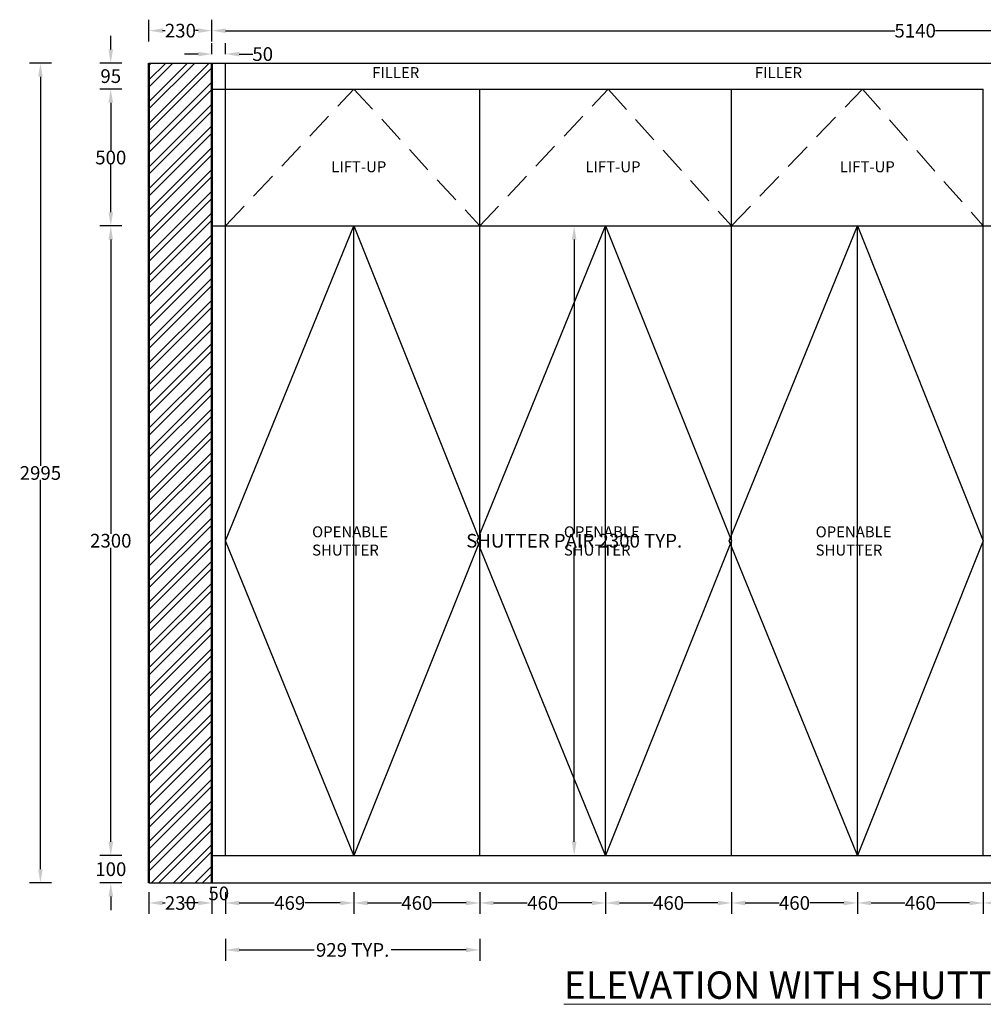
# Model space of a CAD drawing. Units: millimetres. Extents: x -472 to 16192, y -4730 to 4331.
# Tile 1 of 8: x -472 to 3049, y -4730 to -1132. Entities that reach past the tile are written whole.
import ezdxf

# ---------------------------------------------------------------- set-up
doc = ezdxf.new("R2010")
doc.units = ezdxf.units.MM
doc.header["$MEASUREMENT"] = 0
doc.linetypes.add('DASHED', pattern=[0.75, 0.5, -0.25])
for name, color, linetype, lineweight in [('A-ANNO-DIMS', 2, 'Continuous', 18), ('A-ANNO-TEXT', 6, 'Continuous', 18), ('A-ELEV', 7, 'Continuous', 25), ('A-ELEV-SWNG', 4, 'DASHED', 13), ('A-WALL', 7, 'Continuous', 50), ('A-WALL-PATT', 8, 'Continuous', 13)]:
    doc.layers.add(name, color=color, linetype=linetype, lineweight=lineweight)
doc.styles.get("Standard").update_dxf_attribs({"font": 'arial.ttf'})
doc.dimstyles.get("Standard").update_dxf_attribs({"dimtxt": 50, "dimasz": 50, "dimexe": 40, "dimexo": 40, "dimgap": 0.09, "dimtad": 0, "dimtih": 1, "dimtoh": 1, "dimdec": 0, "dimzin": 0, "dimdsep": 46, "dimtxsty": 'Standard', "dimcen": 0.09, "dimclrd": 1, "dimclre": 3, "dimclrt": 6, "dimadec": 0, "dimazin": 0, "dimtfac": 1, "dimtdec": 0, "dimtofl": 0, "dimtmove": 0, "dimatfit": 3, "dimfxl": 40, "dimfxlon": 1, "dimtolj": 1, "dimtzin": 0, "dimarcsym": 0})

# ---------------------------------------------------------------- blocks, each defined once
blk = doc.blocks.new('*D17')
at = {"layer": 'A-ANNO-DIMS', "color": 0, "lineweight": -2, "transparency": 16777216}
for p, q in [((230, -1212.4), (230, -1132.4)), ((5370, -1212.4), (5370, -1132.4)), ((280, -1172.4), (2725.3, -1172.4)), ((5320, -1172.4), (2874.7, -1172.4))]:
    blk.add_line(p, q, dxfattribs=at)
at = {"layer": 'A-ANNO-DIMS', "color": 0, "transparency": 16777216}
for points in [[(280, -1164.1), (280, -1180.8), (230, -1172.4)], [(5320, -1164.1), (5320, -1180.8), (5370, -1172.4)]]:
    blk.add_solid(points, dxfattribs=at)
at = {"layer": 'Defpoints', "color": 0, "transparency": 16777216}
for p in [(5370, -1172.4), (230, -1290.9), (5370, -1290.9)]:
    blk.add_point(p, dxfattribs=at)
at = {"layer": 'A-ANNO-DIMS', "color": 0, "transparency": 16777216, "insert": (2800, -1172.4), "char_height": 50, "attachment_point": 5}
blk.add_mtext('\\A1;5140', dxfattribs=at)
blk = doc.blocks.new('*D19')
at = {"layer": 'A-ANNO-DIMS', "color": 0, "lineweight": -2, "transparency": 16777216}
for p, q in [((230, -1257.8), (230, -1217.8)), ((280, -1257.8), (280, -1217.8)), ((180, -1257.8), (130, -1257.8)), ((330, -1257.8), (380, -1257.8))]:
    blk.add_line(p, q, dxfattribs=at)
at = {"layer": 'A-ANNO-DIMS', "color": 0, "transparency": 16777216}
for points in [[(180, -1249.5), (180, -1266.2), (230, -1257.8)], [(330, -1249.5), (330, -1266.2), (280, -1257.8)]]:
    blk.add_solid(points, dxfattribs=at)
at = {"layer": 'Defpoints', "color": 0, "transparency": 16777216}
for p in [(280, -1257.8), (230, -1290.9), (280, -1290.9)]:
    blk.add_point(p, dxfattribs=at)
at = {"layer": 'A-ANNO-DIMS', "color": 0, "transparency": 16777216, "insert": (415.8, -1257.8), "char_height": 50, "attachment_point": 5}
blk.add_mtext('\\A1;50', dxfattribs=at)
blk = doc.blocks.new('*D20')
at = {"layer": 'A-ANNO-DIMS', "color": 0, "lineweight": -2, "transparency": 16777216}
for p, q in [((0, -1212.3), (0, -1132.3)), ((230, -1212.3), (230, -1132.3)), ((50, -1172.3), (59.3, -1172.3)), ((180, -1172.3), (170.7, -1172.3))]:
    blk.add_line(p, q, dxfattribs=at)
at = {"layer": 'A-ANNO-DIMS', "color": 0, "transparency": 16777216}
for points in [[(50, -1163.9), (50, -1180.6), (0, -1172.3)], [(180, -1163.9), (180, -1180.6), (230, -1172.3)]]:
    blk.add_solid(points, dxfattribs=at)
at = {"layer": 'Defpoints', "color": 0, "transparency": 16777216}
for p in [(230, -1172.3), (0, -1290.9), (230, -1290.9)]:
    blk.add_point(p, dxfattribs=at)
at = {"layer": 'A-ANNO-DIMS', "color": 0, "transparency": 16777216, "insert": (115, -1172.3), "char_height": 50, "attachment_point": 5}
blk.add_mtext('\\A1;230', dxfattribs=at)
blk = doc.blocks.new('*D21')
at = {"layer": 'A-ANNO-DIMS', "color": 0, "lineweight": -2, "transparency": 16777216}
for p, q in [((-356.5, -1290.9), (-436.5, -1290.9)), ((-396.5, -1340.9), (-396.5, -2762.8)), ((-396.5, -4235.9), (-396.5, -2814)), ((-356.5, -4285.9), (-436.5, -4285.9))]:
    blk.add_line(p, q, dxfattribs=at)
at = {"layer": 'A-ANNO-DIMS', "color": 0, "transparency": 16777216}
for points in [[(-404.8, -1340.9), (-388.1, -1340.9), (-396.5, -1290.9)], [(-404.8, -4235.9), (-388.1, -4235.9), (-396.5, -4285.9)]]:
    blk.add_solid(points, dxfattribs=at)
at = {"layer": 'Defpoints', "color": 0, "transparency": 16777216}
for p in [(0, -1290.9), (-396.5, -4285.9), (0, -4285.9)]:
    blk.add_point(p, dxfattribs=at)
at = {"layer": 'A-ANNO-DIMS', "color": 0, "transparency": 16777216, "insert": (-396.5, -2788.4), "char_height": 50, "attachment_point": 5}
blk.add_mtext('\\A1;2995', dxfattribs=at)
blk = doc.blocks.new('*D22')
at = {"layer": 'A-ANNO-DIMS', "color": 0, "lineweight": -2, "transparency": 16777216}
for p, q in [((-139.2, -4135.9), (-139.2, -4085.9)), ((-99.2, -4185.9), (-179.2, -4185.9)), ((-99.2, -4285.9), (-179.2, -4285.9)), ((-139.2, -4335.9), (-139.2, -4385.9))]:
    blk.add_line(p, q, dxfattribs=at)
at = {"layer": 'A-ANNO-DIMS', "color": 0, "transparency": 16777216}
for points in [[(-147.5, -4135.9), (-130.8, -4135.9), (-139.2, -4185.9)], [(-147.5, -4335.9), (-130.8, -4335.9), (-139.2, -4285.9)]]:
    blk.add_solid(points, dxfattribs=at)
at = {"layer": 'Defpoints', "color": 0, "transparency": 16777216}
for p in [(230, -4185.9), (-139.2, -4285.9), (230, -4285.9)]:
    blk.add_point(p, dxfattribs=at)
at = {"layer": 'A-ANNO-DIMS', "color": 0, "transparency": 16777216, "insert": (-139.2, -4235.9), "char_height": 50, "attachment_point": 5}
blk.add_mtext('\\A1;100', dxfattribs=at)
blk = doc.blocks.new('*D23')
at = {"layer": 'A-ANNO-DIMS', "color": 0, "lineweight": -2, "transparency": 16777216}
for p, q in [((-99.4, -1885.9), (-179.4, -1885.9)), ((-139.4, -1935.9), (-139.4, -3010.3)), ((-139.4, -4135.9), (-139.4, -3061.5)), ((-99.4, -4185.9), (-179.4, -4185.9))]:
    blk.add_line(p, q, dxfattribs=at)
at = {"layer": 'A-ANNO-DIMS', "color": 0, "transparency": 16777216}
for points in [[(-147.7, -1935.9), (-131, -1935.9), (-139.4, -1885.9)], [(-147.7, -4135.9), (-131, -4135.9), (-139.4, -4185.9)]]:
    blk.add_solid(points, dxfattribs=at)
at = {"layer": 'Defpoints', "color": 0, "transparency": 16777216}
for p in [(230, -1885.9), (-139.4, -4185.9), (230, -4185.9)]:
    blk.add_point(p, dxfattribs=at)
at = {"layer": 'A-ANNO-DIMS', "color": 0, "transparency": 16777216, "insert": (-139.4, -3035.9), "char_height": 50, "attachment_point": 5}
blk.add_mtext('\\A1;2300', dxfattribs=at)
blk = doc.blocks.new('*D24')
at = {"layer": 'A-ANNO-DIMS', "color": 0, "lineweight": -2, "transparency": 16777216}
for p, q in [((-99.4, -1385.9), (-179.4, -1385.9)), ((-139.4, -1435.9), (-139.4, -1610.3)), ((-139.4, -1835.9), (-139.4, -1661.5)), ((-99.4, -1885.9), (-179.4, -1885.9))]:
    blk.add_line(p, q, dxfattribs=at)
at = {"layer": 'A-ANNO-DIMS', "color": 0, "transparency": 16777216}
for points in [[(-147.7, -1435.9), (-131, -1435.9), (-139.4, -1385.9)], [(-147.7, -1835.9), (-131, -1835.9), (-139.4, -1885.9)]]:
    blk.add_solid(points, dxfattribs=at)
at = {"layer": 'Defpoints', "color": 0, "transparency": 16777216}
for p in [(230, -1385.9), (-139.4, -1885.9), (230, -1885.9)]:
    blk.add_point(p, dxfattribs=at)
at = {"layer": 'A-ANNO-DIMS', "color": 0, "transparency": 16777216, "insert": (-139.4, -1635.9), "char_height": 50, "attachment_point": 5}
blk.add_mtext('\\A1;500', dxfattribs=at)
blk = doc.blocks.new('*D25')
at = {"layer": 'A-ANNO-DIMS', "color": 0, "lineweight": -2, "transparency": 16777216}
for p, q in [((-139.4, -1240.9), (-139.4, -1190.9)), ((-99.4, -1290.9), (-179.4, -1290.9)), ((-99.4, -1385.9), (-179.4, -1385.9)), ((-139.4, -1435.9), (-139.4, -1485.9))]:
    blk.add_line(p, q, dxfattribs=at)
at = {"layer": 'A-ANNO-DIMS', "color": 0, "transparency": 16777216}
for points in [[(-147.7, -1240.9), (-131, -1240.9), (-139.4, -1290.9)], [(-147.7, -1435.9), (-131, -1435.9), (-139.4, -1385.9)]]:
    blk.add_solid(points, dxfattribs=at)
at = {"layer": 'Defpoints', "color": 0, "transparency": 16777216}
for p in [(230, -1290.9), (-139.4, -1385.9), (230, -1385.9)]:
    blk.add_point(p, dxfattribs=at)
at = {"layer": 'A-ANNO-DIMS', "color": 0, "transparency": 16777216, "insert": (-139.4, -1338.4), "char_height": 50, "attachment_point": 5}
blk.add_mtext('\\A1;95', dxfattribs=at)
blk = doc.blocks.new('*D26')
at = {"layer": 'A-ANNO-DIMS', "color": 0, "lineweight": -2, "transparency": 16777216}
for p, q in [((0, -4319.4), (0, -4399.4)), ((230, -4319.4), (230, -4399.4)), ((50, -4359.4), (59.3, -4359.4)), ((180, -4359.4), (170.7, -4359.4))]:
    blk.add_line(p, q, dxfattribs=at)
at = {"layer": 'A-ANNO-DIMS', "color": 0, "transparency": 16777216}
for points in [[(50, -4351), (50, -4367.7), (0, -4359.4)], [(180, -4351), (180, -4367.7), (230, -4359.4)]]:
    blk.add_solid(points, dxfattribs=at)
at = {"layer": 'Defpoints', "color": 0, "transparency": 16777216}
for p in [(0, -4185.9), (230, -4185.9), (230, -4359.4)]:
    blk.add_point(p, dxfattribs=at)
at = {"layer": 'A-ANNO-DIMS', "color": 0, "transparency": 16777216, "insert": (115, -4359.4), "char_height": 50, "attachment_point": 5}
blk.add_mtext('\\A1;230', dxfattribs=at)
blk = doc.blocks.new('*D27')
at = {"layer": 'A-ANNO-DIMS', "color": 0, "lineweight": -2, "transparency": 16777216}
for p, q in [((230, -4319.4), (230, -4399.4)), ((280, -4319.4), (280, -4399.4)), ((180, -4359.4), (130, -4359.4)), ((330, -4359.4), (380, -4359.4))]:
    blk.add_line(p, q, dxfattribs=at)
at = {"layer": 'A-ANNO-DIMS', "color": 0, "transparency": 16777216}
for points in [[(180, -4351), (180, -4367.7), (230, -4359.4)], [(330, -4351), (330, -4367.7), (280, -4359.4)]]:
    blk.add_solid(points, dxfattribs=at)
at = {"layer": 'Defpoints', "color": 0, "transparency": 16777216}
for p in [(230, -4185.9), (280, -4185.9), (280, -4359.4)]:
    blk.add_point(p, dxfattribs=at)
at = {"layer": 'A-ANNO-DIMS', "color": 0, "transparency": 16777216, "insert": (255.3, -4324.5), "char_height": 50, "attachment_point": 5}
blk.add_mtext('\\A1;50', dxfattribs=at)
blk = doc.blocks.new('*D28')
at = {"layer": 'A-ANNO-DIMS', "color": 0, "lineweight": -2, "transparency": 16777216}
for p, q in [((280, -4319.4), (280, -4399.4)), ((749, -4319.4), (749, -4399.4)), ((330, -4359.4), (458.1, -4359.4)), ((699, -4359.4), (570.9, -4359.4))]:
    blk.add_line(p, q, dxfattribs=at)
at = {"layer": 'A-ANNO-DIMS', "color": 0, "transparency": 16777216}
for points in [[(330, -4351), (330, -4367.7), (280, -4359.4)], [(699, -4351), (699, -4367.7), (749, -4359.4)]]:
    blk.add_solid(points, dxfattribs=at)
at = {"layer": 'Defpoints', "color": 0, "transparency": 16777216}
for p in [(280, -4185.9), (749, -4185.9), (749, -4359.4)]:
    blk.add_point(p, dxfattribs=at)
at = {"layer": 'A-ANNO-DIMS', "color": 0, "transparency": 16777216, "insert": (514.5, -4359.4), "char_height": 50, "attachment_point": 5}
blk.add_mtext('\\A1;469', dxfattribs=at)
blk = doc.blocks.new('*D29')
at = {"layer": 'A-ANNO-DIMS', "color": 0, "lineweight": -2, "transparency": 16777216}
for p, q in [((749, -4319.4), (749, -4399.4)), ((1209, -4319.4), (1209, -4399.4)), ((799, -4359.4), (922.8, -4359.4)), ((1159, -4359.4), (1035.2, -4359.4))]:
    blk.add_line(p, q, dxfattribs=at)
at = {"layer": 'A-ANNO-DIMS', "color": 0, "transparency": 16777216}
for points in [[(799, -4351), (799, -4367.7), (749, -4359.4)], [(1159, -4351), (1159, -4367.7), (1209, -4359.4)]]:
    blk.add_solid(points, dxfattribs=at)
at = {"layer": 'Defpoints', "color": 0, "transparency": 16777216}
for p in [(749, -4185.9), (1209, -4185.9), (1209, -4359.4)]:
    blk.add_point(p, dxfattribs=at)
at = {"layer": 'A-ANNO-DIMS', "color": 0, "transparency": 16777216, "insert": (979, -4359.4), "char_height": 50, "attachment_point": 5}
blk.add_mtext('\\A1;460', dxfattribs=at)
blk = doc.blocks.new('*D30')
at = {"layer": 'A-ANNO-DIMS', "color": 0, "lineweight": -2, "transparency": 16777216}
for p, q in [((1209, -4319.4), (1209, -4399.4)), ((1669, -4319.4), (1669, -4399.4)), ((1259, -4359.4), (1382.8, -4359.4)), ((1619, -4359.4), (1495.2, -4359.4))]:
    blk.add_line(p, q, dxfattribs=at)
at = {"layer": 'A-ANNO-DIMS', "color": 0, "transparency": 16777216}
for points in [[(1259, -4351), (1259, -4367.7), (1209, -4359.4)], [(1619, -4351), (1619, -4367.7), (1669, -4359.4)]]:
    blk.add_solid(points, dxfattribs=at)
at = {"layer": 'Defpoints', "color": 0, "transparency": 16777216}
for p in [(1209, -4185.9), (1669, -4185.9), (1669, -4359.4)]:
    blk.add_point(p, dxfattribs=at)
at = {"layer": 'A-ANNO-DIMS', "color": 0, "transparency": 16777216, "insert": (1439, -4359.4), "char_height": 50, "attachment_point": 5}
blk.add_mtext('\\A1;460', dxfattribs=at)
blk = doc.blocks.new('*D31')
at = {"layer": 'A-ANNO-DIMS', "color": 0, "lineweight": -2, "transparency": 16777216}
for p, q in [((1669, -4319.4), (1669, -4399.4)), ((2129, -4319.4), (2129, -4399.4)), ((1719, -4359.4), (1842.8, -4359.4)), ((2079, -4359.4), (1955.2, -4359.4))]:
    blk.add_line(p, q, dxfattribs=at)
at = {"layer": 'A-ANNO-DIMS', "color": 0, "transparency": 16777216}
for points in [[(1719, -4351), (1719, -4367.7), (1669, -4359.4)], [(2079, -4351), (2079, -4367.7), (2129, -4359.4)]]:
    blk.add_solid(points, dxfattribs=at)
at = {"layer": 'Defpoints', "color": 0, "transparency": 16777216}
for p in [(1669, -4185.9), (2129, -4185.9), (2129, -4359.4)]:
    blk.add_point(p, dxfattribs=at)
at = {"layer": 'A-ANNO-DIMS', "color": 0, "transparency": 16777216, "insert": (1899, -4359.4), "char_height": 50, "attachment_point": 5}
blk.add_mtext('\\A1;460', dxfattribs=at)
blk = doc.blocks.new('*D32')
at = {"layer": 'A-ANNO-DIMS', "color": 0, "lineweight": -2, "transparency": 16777216}
for p, q in [((2129, -4319.4), (2129, -4399.4)), ((2589, -4319.4), (2589, -4399.4)), ((2179, -4359.4), (2302.8, -4359.4)), ((2539, -4359.4), (2415.2, -4359.4))]:
    blk.add_line(p, q, dxfattribs=at)
at = {"layer": 'A-ANNO-DIMS', "color": 0, "transparency": 16777216}
for points in [[(2179, -4351), (2179, -4367.7), (2129, -4359.4)], [(2539, -4351), (2539, -4367.7), (2589, -4359.4)]]:
    blk.add_solid(points, dxfattribs=at)
at = {"layer": 'Defpoints', "color": 0, "transparency": 16777216}
for p in [(2129, -4185.9), (2589, -4185.9), (2589, -4359.4)]:
    blk.add_point(p, dxfattribs=at)
at = {"layer": 'A-ANNO-DIMS', "color": 0, "transparency": 16777216, "insert": (2359, -4359.4), "char_height": 50, "attachment_point": 5}
blk.add_mtext('\\A1;460', dxfattribs=at)
blk = doc.blocks.new('*D33')
at = {"layer": 'A-ANNO-DIMS', "color": 0, "lineweight": -2, "transparency": 16777216}
for p, q in [((2589, -4319.4), (2589, -4399.4)), ((3049, -4319.4), (3049, -4399.4)), ((2639, -4359.4), (2762.8, -4359.4)), ((2999, -4359.4), (2875.2, -4359.4))]:
    blk.add_line(p, q, dxfattribs=at)
at = {"layer": 'A-ANNO-DIMS', "color": 0, "transparency": 16777216}
for points in [[(2639, -4351), (2639, -4367.7), (2589, -4359.4)], [(2999, -4351), (2999, -4367.7), (3049, -4359.4)]]:
    blk.add_solid(points, dxfattribs=at)
at = {"layer": 'Defpoints', "color": 0, "transparency": 16777216}
for p in [(2589, -4185.9), (3049, -4185.9), (3049, -4359.4)]:
    blk.add_point(p, dxfattribs=at)
at = {"layer": 'A-ANNO-DIMS', "color": 0, "transparency": 16777216, "insert": (2819, -4359.4), "char_height": 50, "attachment_point": 5}
blk.add_mtext('\\A1;460', dxfattribs=at)
blk = doc.blocks.new('*D34')
at = {"layer": 'A-ANNO-DIMS', "color": 0, "lineweight": -2, "transparency": 16777216}
for p, q in [((3049, -4319.4), (3049, -4399.4)), ((3509, -4319.4), (3509, -4399.4)), ((3099, -4359.4), (3222.8, -4359.4)), ((3459, -4359.4), (3335.2, -4359.4))]:
    blk.add_line(p, q, dxfattribs=at)
at = {"layer": 'A-ANNO-DIMS', "color": 0, "transparency": 16777216}
for points in [[(3099, -4351), (3099, -4367.7), (3049, -4359.4)], [(3459, -4351), (3459, -4367.7), (3509, -4359.4)]]:
    blk.add_solid(points, dxfattribs=at)
at = {"layer": 'Defpoints', "color": 0, "transparency": 16777216}
for p in [(3049, -4185.9), (3509, -4185.9), (3509, -4359.4)]:
    blk.add_point(p, dxfattribs=at)
at = {"layer": 'A-ANNO-DIMS', "color": 0, "transparency": 16777216, "insert": (3279, -4359.4), "char_height": 50, "attachment_point": 5}
blk.add_mtext('\\A1;460', dxfattribs=at)
blk = doc.blocks.new('SHUTTER-PAIR')
at = {"ltscale": 200}
for p, q in [((0, 1150), (469, 2300)), ((469, 2300), (929, 1150)), ((469, 0), (0, 1150)), ((929, 1150), (469, 0))]:
    blk.add_line(p, q, dxfattribs=at)
blk.add_line((469, 0), (469, 2300))
blk = doc.blocks.new('*D93')
at = {"layer": 'A-ANNO-DIMS', "color": 3, "lineweight": -2, "transparency": 16777216}
for p, q in [((1514, -1885.9), (1594, -1885.9)), ((1514, -4185.9), (1594, -4185.9))]:
    blk.add_line(p, q, dxfattribs=at)
at = {"layer": 'A-ANNO-DIMS', "color": 1, "lineweight": -2, "transparency": 16777216}
for p, q in [((1554, -1935.9), (1554, -3009.9)), ((1554, -4135.9), (1554, -3061.9))]:
    blk.add_line(p, q, dxfattribs=at)
at = {"layer": 'A-ANNO-DIMS', "color": 1, "transparency": 16777216}
for points in [[(1545.7, -1935.9), (1562.3, -1935.9), (1554, -1885.9)], [(1545.7, -4135.9), (1562.3, -4135.9), (1554, -4185.9)]]:
    blk.add_solid(points, dxfattribs=at)
at = {"layer": 'Defpoints', "color": 0, "transparency": 16777216}
for p in [(1209, -1885.9), (1554, -1885.9), (1209, -4185.9)]:
    blk.add_point(p, dxfattribs=at)
at = {"layer": 'A-ANNO-DIMS', "color": 6, "transparency": 16777216, "insert": (1554, -3035.9), "char_height": 50, "attachment_point": 5}
blk.add_mtext('\\A1;SHUTTER PAIR 2300 TYP.', dxfattribs=at)
blk = doc.blocks.new('*D94')
at = {"layer": 'A-ANNO-DIMS', "color": 3, "lineweight": -2, "transparency": 16777216}
for p, q in [((280, -4490.9), (280, -4570.9)), ((1209, -4490.9), (1209, -4570.9))]:
    blk.add_line(p, q, dxfattribs=at)
at = {"layer": 'A-ANNO-DIMS', "color": 1, "lineweight": -2, "transparency": 16777216}
for p, q in [((330, -4530.9), (603.3, -4530.9)), ((1159, -4530.9), (885.7, -4530.9))]:
    blk.add_line(p, q, dxfattribs=at)
at = {"layer": 'A-ANNO-DIMS', "color": 1, "transparency": 16777216}
for points in [[(330, -4522.6), (330, -4539.2), (280, -4530.9)], [(1159, -4522.6), (1159, -4539.2), (1209, -4530.9)]]:
    blk.add_solid(points, dxfattribs=at)
at = {"layer": 'Defpoints', "color": 0, "transparency": 16777216}
for p in [(280, -4185.9), (1209, -4185.9), (1209, -4530.9)]:
    blk.add_point(p, dxfattribs=at)
at = {"layer": 'A-ANNO-DIMS', "color": 6, "transparency": 16777216, "insert": (744.5, -4530.9), "char_height": 50, "attachment_point": 5}
blk.add_mtext('\\A1;929 TYP.', dxfattribs=at)

msp = doc.modelspace()

# ---------------------------------------------------------------- hatches: boundary and pattern name
at = {"layer": 'A-WALL-PATT'}
h = msp.add_hatch(dxfattribs=at)
h.set_pattern_fill('ANSI32', color=256, scale=150)
h.paths.add_polyline_path([(9720.7, -1290.9), (9720.7, -4285.9), (9950.7, -4285.9), (9950.7, -4185.9), (9950.7, -1885.9), (9950.7, -1290.9)])
h.paths.add_polyline_path([(5370, -4285.9), (5600, -4285.9), (5600, -1290.9), (5370, -1290.9)])
h.paths.add_polyline_path([(15320.7, -1290.9), (15090.7, -1290.9), (15090.7, -4285.9), (15320.7, -4285.9)])
h.paths.add_polyline_path([(0, -4285.9), (230, -4285.9), (230, -4185.9), (230, -1885.9), (230, -1290.9), (0, -1290.9)])

# ---------------------------------------------------------------- linework, layer by layer
at = {"layer": 'A-ELEV'}
for p, q in [((0, -1290.9), (5600, -1290.9)), ((280, -4185.9), (280, -1290.9)), ((230, -1385.9), (3049, -1385.9)), ((1209, -4185.9), (1209, -1385.9)), ((2129, -4185.9), (2129, -1385.9)), ((3049, -1885.9), (3049, -1385.9)), ((230, -1885.9), (5370, -1885.9)), ((3049, -4185.9), (3049, -1885.9)), ((230, -4185.9), (3509, -4185.9)), ((0, -4285.9), (5600, -4285.9))]:
    msp.add_line(p, q, dxfattribs=at)
at = {"layer": 'A-ELEV-SWNG', "ltscale": 200}
for p, q in [((280, -1885.9), (749, -1385.9)), ((749, -1385.9), (1209, -1885.9)), ((1209, -1885.9), (1678, -1385.9)), ((1678, -1385.9), (2129, -1885.9)), ((2129, -1885.9), (2607, -1385.9)), ((2607, -1385.9), (3049, -1885.9))]:
    msp.add_line(p, q, dxfattribs=at)
at = {"layer": 'A-WALL'}
for p, q in [((0, -4285.9), (0, -1290.9)), ((230, -1885.9), (230, -1290.9)), ((230, -4185.9), (230, -1885.9)), ((230, -4285.9), (230, -4185.9))]:
    msp.add_line(p, q, dxfattribs=at)

# ---------------------------------------------------------------- block references
at = {"layer": 'A-ELEV'}
for p in [(280, -4185.9), (1200, -4185.9), (2120, -4185.9)]:
    msp.add_blockref('SHUTTER-PAIR', p, dxfattribs=at)

# ---------------------------------------------------------------- texts
at = {"layer": 'A-ANNO-TEXT', "attachment_point": 1}
for s, width, insert, char_height in [('FILLER', 327.678, (815.8, -1305.7), 40), ('FILLER', 327.678, (2214.5, -1305.7), 40), ('LIFT-UP', 327.678, (666.2, -1649.6), 40), ('LIFT-UP', 327.678, (1595.2, -1649.6), 40), ('LIFT-UP', 327.678, (2524.2, -1649.6), 40), ('OPENABLE \\PSHUTTER', 327.678, (596.3, -2983.4), 40), ('OPENABLE \\PSHUTTER', 327.678, (1516.3, -2983.4), 40), ('OPENABLE \\PSHUTTER', 327.678, (2436.3, -2983.4), 40), ('{\\fArial|b1|i0|c0|p34;\\LELEVATION WITH SHUTTER}', 3435.915, (1516.3, -4609.6), 100)]:
    msp.add_mtext_dynamic_manual_height_columns(s, width=width, gutter_width=1, heights=[0], dxfattribs=dict(at, insert=insert, char_height=char_height))

# ---------------------------------------------------------------- dimensions: what is measured, and where the dimension line sits
at = {"layer": 'A-ANNO-DIMS'}
for base, p1, p2, override, picture, middle in [((230, -1172.3), (0, -1290.9), (230, -1290.9), {"dimclrd": 0, "dimclre": 0, "dimclrt": 0}, '*D20', (115, -1172.3)), ((5370, -1172.4), (230, -1290.9), (5370, -1290.9), {"dimclrd": 0, "dimclre": 0, "dimclrt": 0}, '*D17', (2800, -1172.4)), ((280, -1257.8), (230, -1290.9), (280, -1290.9), {"dimclrd": 0, "dimclre": 0, "dimclrt": 0}, '*D19', (415.8, -1257.8)), ((230, -4359.4), (0, -4185.9), (230, -4185.9), {"dimclrd": 0, "dimclre": 0, "dimclrt": 0}, '*D26', (115, -4359.4)), ((749, -4359.4), (280, -4185.9), (749, -4185.9), {"dimclrd": 0, "dimclre": 0, "dimclrt": 0, "dimtmove": 1}, '*D28', (514.5, -4359.4)), ((1209, -4359.4), (749, -4185.9), (1209, -4185.9), {"dimclrd": 0, "dimclre": 0, "dimclrt": 0, "dimtmove": 1}, '*D29', (979, -4359.4)), ((1669, -4359.4), (1209, -4185.9), (1669, -4185.9), {"dimclrd": 0, "dimclre": 0, "dimclrt": 0, "dimtmove": 1}, '*D30', (1439, -4359.4)), ((2129, -4359.4), (1669, -4185.9), (2129, -4185.9), {"dimclrd": 0, "dimclre": 0, "dimclrt": 0, "dimtmove": 1}, '*D31', (1899, -4359.4)), ((2589, -4359.4), (2129, -4185.9), (2589, -4185.9), {"dimclrd": 0, "dimclre": 0, "dimclrt": 0, "dimtmove": 1}, '*D32', (2359, -4359.4)), ((3049, -4359.4), (2589, -4185.9), (3049, -4185.9), {"dimclrd": 0, "dimclre": 0, "dimclrt": 0, "dimtmove": 1}, '*D33', (2819, -4359.4)), ((3509, -4359.4), (3049, -4185.9), (3509, -4185.9), {"dimclrd": 0, "dimclre": 0, "dimclrt": 0, "dimtmove": 1}, '*D34', (3279, -4359.4))]:
    dim = msp.add_linear_dim(base=base, p1=p1, p2=p2, dimstyle='Standard', override=override, dxfattribs=at)
    dim.commit()
    dim.dimension.update_dxf_attribs({"geometry": picture, "text_midpoint": middle})
for base, p1, p2, picture, middle in [((-139.4, -1385.9), (230, -1290.9), (230, -1385.9), '*D25', (-139.4, -1338.4)), ((-396.5, -4285.9), (0, -1290.9), (0, -4285.9), '*D21', (-396.5, -2788.4)), ((-139.4, -1885.9), (230, -1385.9), (230, -1885.9), '*D24', (-139.4, -1635.9)), ((-139.4, -4185.9), (230, -1885.9), (230, -4185.9), '*D23', (-139.4, -3035.9)), ((-139.2, -4285.9), (230, -4185.9), (230, -4285.9), '*D22', (-139.2, -4235.9))]:
    dim = msp.add_linear_dim(base=base, p1=p1, p2=p2, angle=90, dimstyle='Standard', override={"dimclrd": 0, "dimclre": 0, "dimclrt": 0}, dxfattribs=at)
    dim.commit()
    dim.dimension.update_dxf_attribs({"geometry": picture, "text_midpoint": middle})
dim = msp.add_linear_dim(base=(1554, -1885.9), p1=(1209, -4185.9), p2=(1209, -1885.9), angle=90, text='SHUTTER PAIR <> TYP.', dimstyle='Standard', override={"dimdec": 0, "dimrnd": 0, "dimzin": 0, "dimlunit": 2}, dxfattribs=at)
dim.commit()
dim.dimension.update_dxf_attribs({"geometry": '*D93', "text_midpoint": (1554, -3035.9)})
dim = msp.add_linear_dim(base=(280, -4359.4), p1=(230, -4185.9), p2=(280, -4185.9), dimstyle='Standard', override={"dimclrd": 0, "dimclre": 0, "dimclrt": 0, "dimtmove": 2}, dxfattribs=at)
dim.commit()
dim.dimension.update_dxf_attribs({"geometry": '*D27', "text_midpoint": (255.3, -4324.5), "dimtype": 160})
dim = msp.add_linear_dim(base=(1209, -4530.9), p1=(280, -4185.9), p2=(1209, -4185.9), text='<> TYP.', dimstyle='Standard', override={"dimdec": 0, "dimrnd": 0, "dimzin": 0, "dimlunit": 2}, dxfattribs=at)
dim.commit()
dim.dimension.update_dxf_attribs({"geometry": '*D94', "text_midpoint": (744.5, -4530.9)})

doc.saveas('drawing.dxf')
